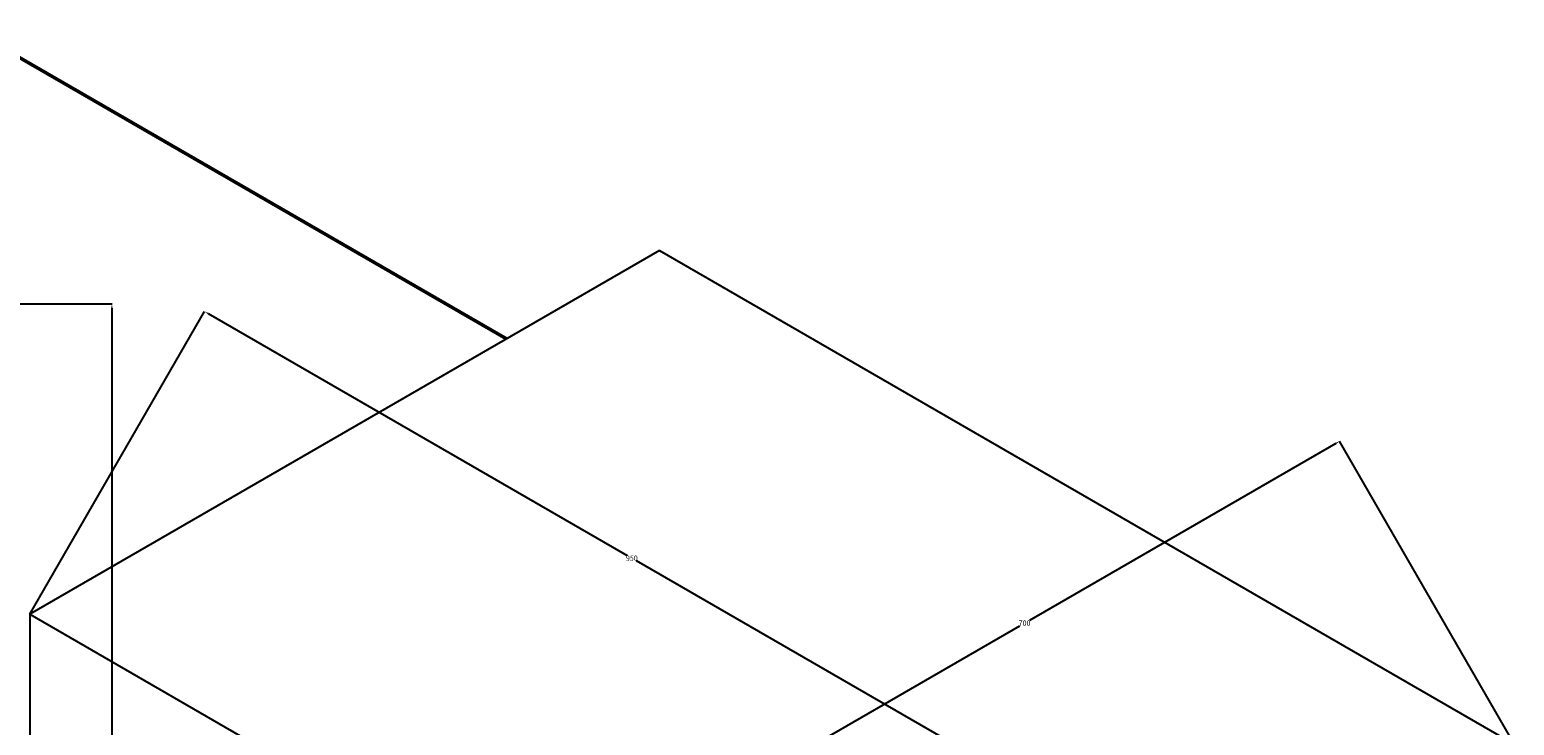
# Model space of a CAD drawing. Units: metres. Extents: x -2391 to 4922, y -635 to 4845.
# Tile 37 of 37: x 3149 to 4578, y 2368 to 3038. Entities that reach past the tile are written whole.
import ezdxf

# ---------------------------------------------------------------- set-up
doc = ezdxf.new("R2010")
doc.units = ezdxf.units.M
doc.header["$MEASUREMENT"] = 0
for name, color, linetype, lineweight in [('A-ANNO-DIMS', 2, 'Continuous', 18), ('A-FLOR-FIXT', 3, 'Continuous', 25), ('A-WALL', 7, 'Continuous', 50)]:
    doc.layers.add(name, color=color, linetype=linetype, lineweight=lineweight)
doc.styles.get("Standard").update_dxf_attribs({"font": 'arial.ttf'})
doc.dimstyles.get("Standard").update_dxf_attribs({"dimtxt": 5, "dimasz": 4, "dimexe": 0.18, "dimexo": 0.0625, "dimgap": 0.09, "dimtad": 0, "dimtih": 1, "dimtoh": 1, "dimdec": 0, "dimzin": 0, "dimdsep": 46, "dimtxsty": 'Standard', "dimcen": 0.09, "dimadec": 0, "dimazin": 0, "dimtfac": 1, "dimtdec": 0, "dimtofl": 0, "dimtmove": 0, "dimatfit": 3, "dimfxl": 1, "dimtolj": 1, "dimtzin": 0, "dimarcsym": 0})

# ---------------------------------------------------------------- blocks, each defined once
blk = doc.blocks.new('*D8')
at = {"layer": 'A-ANNO-DIMS', "color": 0, "lineweight": -2, "transparency": 16777216}
for p, q in [((-2047.3, 3005.2), (-2047.3, -631.4)), ((4577.8, 2350.2), (4577.8, -631.4)), ((-2043.3, -631.2), (1257.6, -631.2)), ((4573.8, -631.2), (1272.8, -631.2))]:
    blk.add_line(p, q, dxfattribs=at)
at = {"layer": 'A-ANNO-DIMS', "color": 0, "transparency": 16777216}
for points in [[(-2043.3, -630.6), (-2043.3, -631.9), (-2047.3, -631.2)], [(4573.8, -630.6), (4573.8, -631.9), (4577.8, -631.2)]]:
    blk.add_solid(points, dxfattribs=at)
at = {"layer": 'Defpoints', "color": 0, "transparency": 16777216}
for p in [(-2047.3, 3005.3), (4577.8, 2350.3), (4577.8, -631.2)]:
    blk.add_point(p, dxfattribs=at)
at = {"layer": 'A-ANNO-DIMS', "color": 0, "transparency": 16777216, "insert": (1265.2, -631.2), "char_height": 5, "attachment_point": 5}
blk.add_mtext('\\A1;6625', dxfattribs=at)
blk = doc.blocks.new('*D13')
at = {"layer": 'A-ANNO-DIMS', "color": 0, "lineweight": -2, "transparency": 16777216}
for p, q in [((2891.5, 2774), (3228.1, 2774)), ((3227.9, 2770), (3227.9, 2318)), ((3227.9, 1860.8), (3227.9, 2312.8)), ((2891.5, 1856.8), (3228.1, 1856.8))]:
    blk.add_line(p, q, dxfattribs=at)
at = {"layer": 'A-ANNO-DIMS', "color": 0, "transparency": 16777216}
for points in [[(3227.3, 2770), (3228.6, 2770), (3227.9, 2774)], [(3227.3, 1860.8), (3228.6, 1860.8), (3227.9, 1856.8)]]:
    blk.add_solid(points, dxfattribs=at)
at = {"layer": 'Defpoints', "color": 0, "transparency": 16777216}
for p in [(2891.4, 2774), (2891.4, 1856.8), (3227.9, 1856.8)]:
    blk.add_point(p, dxfattribs=at)
at = {"layer": 'A-ANNO-DIMS', "color": 0, "transparency": 16777216, "insert": (3227.9, 2315.4), "char_height": 5, "attachment_point": 5}
blk.add_mtext('\\A1;917.2', dxfattribs=at)
blk = doc.blocks.new('*D28')
at = {"layer": 'A-ANNO-DIMS', "color": 0, "lineweight": -2, "transparency": 16777216}
for p, q in [((3148.8, 2475.3), (3317.2, 2766.8)), ((3320.5, 2764.7), (3723.9, 2531.8)), ((4136.3, 2293.7), (3733, 2526.6)), ((3971.6, 2000.3), (4139.9, 2291.8))]:
    blk.add_line(p, q, dxfattribs=at)
at = {"layer": 'A-ANNO-DIMS', "color": 0, "transparency": 16777216}
for points in [[(3320.9, 2765.3), (3320.2, 2764.1), (3317.1, 2766.7)], [(4136.7, 2294.3), (4136, 2293.1), (4139.8, 2291.7)]]:
    blk.add_solid(points, dxfattribs=at)
at = {"layer": 'Defpoints', "color": 0, "transparency": 16777216}
for p in [(3148.8, 2475.3), (4139.8, 2291.7), (3971.5, 2000.3)]:
    blk.add_point(p, dxfattribs=at)
at = {"layer": 'A-ANNO-DIMS', "color": 0, "transparency": 16777216, "insert": (3728.4, 2529.2), "char_height": 5, "attachment_point": 5}
blk.add_mtext('\\A1;950', dxfattribs=at)
blk = doc.blocks.new('*D29')
at = {"layer": 'A-ANNO-DIMS', "color": 0, "lineweight": -2, "transparency": 16777216}
for p, q in [((4406, 2639.7), (4111, 2469.3)), ((4577.7, 2350.3), (4409.4, 2641.8)), ((3806.8, 2293.7), (4101.8, 2464.1)), ((3971.5, 2000.3), (3803.2, 2291.8))]:
    blk.add_line(p, q, dxfattribs=at)
at = {"layer": 'A-ANNO-DIMS', "color": 0, "transparency": 16777216}
for points in [[(4405.7, 2640.3), (4406.4, 2639.1), (4409.5, 2641.7)], [(3806.4, 2294.3), (3807.1, 2293.1), (3803.3, 2291.7)]]:
    blk.add_solid(points, dxfattribs=at)
at = {"layer": 'Defpoints', "color": 0, "transparency": 16777216}
for p in [(4409.5, 2641.7), (4577.8, 2350.3), (3971.5, 2000.3)]:
    blk.add_point(p, dxfattribs=at)
at = {"layer": 'A-ANNO-DIMS', "color": 0, "transparency": 16777216, "insert": (4106.4, 2466.7), "char_height": 5, "attachment_point": 5}
blk.add_mtext('\\A1;700', dxfattribs=at)

msp = doc.modelspace()

# ---------------------------------------------------------------- linework, layer by layer
at = {"layer": 'A-FLOR-FIXT'}
for p, q in [((3755.0359, 2825.2763), (3148.8181, 2475.2763)), ((3755.0359, 2825.2763), (4577.76, 2350.2763)), ((3148.8181, 2475.2763), (3148.8181, 1505.2763)), ((3148.8181, 2475.2763), (3971.5422, 2000.2763))]:
    msp.add_line(p, q, dxfattribs=at)
at = {"layer": 'A-WALL'}
msp.add_line((550.7419, 4505.2763), (3607.8116, 2740.2763), dxfattribs=at)

# ---------------------------------------------------------------- dimensions: what is measured, and where the dimension line sits
at = {"layer": 'A-ANNO-DIMS'}
dim = msp.add_linear_dim(base=(4577.76, -631.2237), p1=(-2047.3343, 3005.2763), p2=(4577.76, 2350.2763), dimstyle='Standard', override={"dimdec": 0, "dimlfac": 1, "dimrnd": 0, "dimzin": 0, "dimdsep": 46, "dimlunit": 2}, dxfattribs=at)
dim.commit()
dim.dimension.update_dxf_attribs({"geometry": '*D8', "text_midpoint": (1265.2128, -631.2237)})
for base, p1, p2, angle, override, picture, middle in [((3227.9324, 1856.8211), (2891.4324, 2773.9801), (2891.4324, 1856.8211), 270, {"dimdec": 1, "dimlfac": 1, "dimrnd": 0, "dimzin": 0, "dimdsep": 46, "dimlunit": 2}, '*D13', (3227.9324, 2315.4006)), ((4139.7922, 2291.6938), (3148.8181, 2475.2763), (3971.5422, 2000.2763), 330, {"dimdec": 0, "dimlfac": 1, "dimrnd": 0, "dimzin": 0, "dimdsep": 46, "dimlunit": 2}, '*D28', (3728.4302, 2529.1938)), ((4409.51, 2641.6938), (3971.5422, 2000.2763), (4577.76, 2350.2763), 30, {"dimdec": 0, "dimlfac": 1, "dimrnd": 0, "dimzin": 0, "dimdsep": 46, "dimlunit": 2}, '*D29', (4106.4011, 2466.6938))]:
    dim = msp.add_linear_dim(base=base, p1=p1, p2=p2, angle=angle, dimstyle='Standard', override=override, dxfattribs=at)
    dim.commit()
    dim.dimension.update_dxf_attribs({"geometry": picture, "text_midpoint": middle})

doc.saveas('drawing.dxf')
